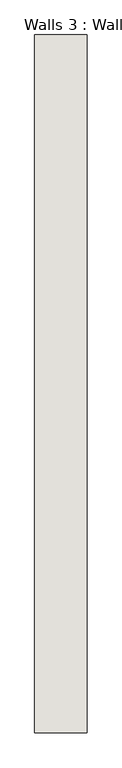
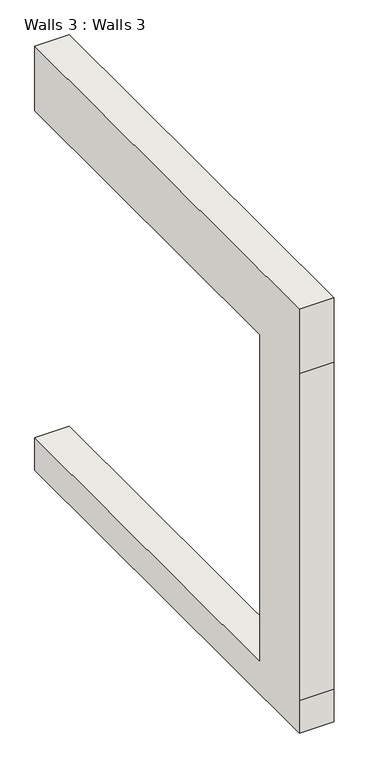
"""IFC4 building model written with IfcOpenShell, lengths in millimetres: wall geometry, Walls 3 : Walls 3."""

from ifc_helpers import new_model, si_unit, frame, origin, place, context, project, spatial, polyline, outline, extrude, source, transform, mapped, element, save


def walls_3_walls_3_63c7a103(model_context):
    return source(origin(), model_context, "Body", "SweptSolid", [
        extrude(outline(polyline([(3667.9425923, 7620.0), (3667.9425923, 7017.1841049), (220.7992188, 7017.1841049), (220.7992188, 3962.4), (3667.9425923, 3962.4), (3667.9425923, 3661.3007362), (-383.6118819, 3661.3007362), (-383.6118819, 3962.4), (-383.6118819, 7017.1841049), (-383.6118819, 7620.0), (3667.9425923, 7620.0)])), frame((-13053.811895, 0.0, 0.0), z_axis=(1.0, 0.0, 0.0), x_axis=(0.0, 1.0, 0.0)), (0.0, 0.0, 1.0), 304.8),
    ])


if __name__ == "__main__":
    model = new_model("IFC4")
    model_context = context("Model", 3, world=origin())
    ifc_project = project(units=[si_unit("LENGTHUNIT", "METRE", prefix="MILLI")], contexts=[model_context])
    site = spatial("IfcSite", under=ifc_project)
    building = spatial("IfcBuilding", under=site)
    placement = place(None, origin())
    walls_3_walls_3_shape = walls_3_walls_3_63c7a103(model_context)
    element("IfcWall", 1, ObjectType="Walls 3 : Walls 3", at=placement, inside=building, context=model_context, shape_type="MappedRepresentation", body=[
        mapped(walls_3_walls_3_shape, transform((0.0, 0.0, 0.0), x_axis=(1.0, 0.0, 0.0), y_axis=(0.0, 1.0, 0.0), z_axis=(0.0, 0.0, 1.0))),
    ])
    save(model, "model.ifc")

# Revit data of these elements
# Element 1 (IfcWall, "Walls 3 : Walls 3")
#   Materials on its faces: "Default Wall"
# Materials
#   "Default Wall": colour RGB 128 128 128, transparency 0
